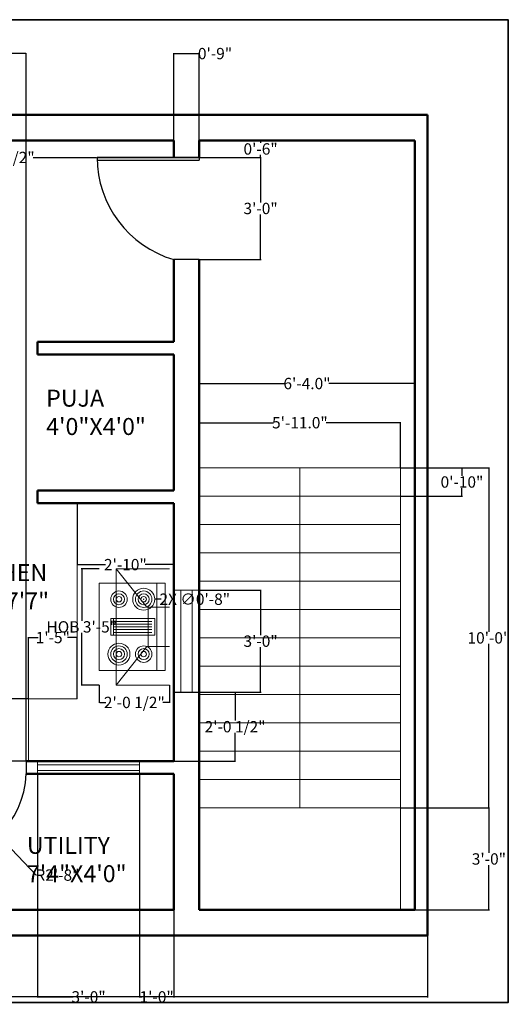
# Model space of a CAD drawing. Units: inches. Extents: x 124 to 591, y 365 to 713.
# Tile 5 of 5: x 418 to 591, y 365 to 713. Entities that reach past the tile are written whole.
import ezdxf

# ---------------------------------------------------------------- set-up
doc = ezdxf.new("R2010")
doc.units = ezdxf.units.IN
doc.header["$MEASUREMENT"] = 0
for name, color, linetype, lineweight in [('A-ANNO-DIMS', 2, 'Continuous', 18), ('A-ANNO-TTLB', 7, 'Continuous', 35), ('A-AREA-IDEN', 7, 'Continuous', 25), ('A-DOOR', 4, 'Continuous', 25), ('A-EQPM', 8, 'Continuous', 18), ('A-FLOR-CASE', 8, 'Continuous', 18), ('A-FLOR-STRS', 7, 'Continuous', 18), ('A-GLAZ', 4, 'Continuous', 18), ('A-WALL', 7, 'Continuous', 50)]:
    doc.layers.add(name, color=color, linetype=linetype, lineweight=lineweight)
doc.styles.get("Standard").update_dxf_attribs({"font": 'arial.ttf'})
doc.dimstyles.get("Standard").update_dxf_attribs({"dimtxt": 4, "dimasz": 0.18, "dimexe": 0.18, "dimexo": 0.0625, "dimgap": 0.09, "dimtad": 0, "dimtih": 1, "dimtoh": 1, "dimdec": 1, "dimzin": 0, "dimdsep": 46, "dimlunit": 3, "dimtxsty": 'Standard', "dimcen": 0.09, "dimclrd": 6, "dimclrt": 3, "dimadec": 0, "dimazin": 0, "dimtfac": 1, "dimtdec": 1, "dimtofl": 0, "dimtmove": 0, "dimatfit": 3, "dimfxl": 1, "dimtfillclr": 6, "dimtolj": 1, "dimtzin": 0, "dimarcsym": 0})

# ---------------------------------------------------------------- blocks, each defined once
blk = doc.blocks.new('chimmne')
for p, q in [((17.89, 6.07), (-18.11, 6.07)), ((-18.11, 6.07), (-18.11, -10.43)), ((-6.16, -3.43), (-18.11, 6.07)), ((5.94, -3.43), (17.89, 6.07)), ((17.89, 6.07), (17.89, -10.43)), ((-6.16, -3.43), (-6.16, -10.43)), ((5.94, -3.82), (-6.16, -3.82)), ((5.94, -3.43), (5.94, -10.43))]:
    blk.add_line(p, q)
for points in [[(-13.61, -9.12), (-13.61, 11.28), (13.39, 11.28), (13.39, -9.12)], [(-2.66, -5.87), (-2.66, 7.73), (2.44, 7.73), (2.44, -5.87)]]:
    blk.add_lwpolyline(points, close=True)
for points in [[(-2.66, 6.88), (2.44, 6.88)], [(-1.81, 6.88), (-1.81, -5.02)], [(-0.96, -5.02), (-0.96, 6.88)], [(-0.11, 6.88), (-0.11, -5.02)], [(0.74, -5.02), (0.74, 6.88)], [(1.59, 6.88), (1.59, -5.02)], [(13.39, -6.57), (-13.61, -6.57)]]:
    blk.add_lwpolyline(points)
for centre, radius in [((-8.55, 5.18), 3.4), ((-8.55, 5.18), 2.55), ((-8.55, 5.18), 1.7), ((8.44, 5.18), 2.55), ((8.44, 5.18), 1.7), ((-8.55, 5.18), 0.85), ((8.44, 5.18), 0.85), ((-8.55, -2.47), 2.55), ((8.44, -2.47), 3.4), ((8.44, -2.47), 2.55), ((-8.55, -2.47), 1.7), ((-8.55, -2.47), 0.85), ((8.44, -2.47), 1.7), ((8.44, -2.47), 0.85)]:
    blk.add_circle(centre, radius)
blk = doc.blocks.new('*D22')
at = {"layer": 'A-ANNO-DIMS', "color": 0, "lineweight": -2, "transparency": 16777216}
for p, q in [((481.64, 554.65), (481.64, 570.69)), ((481.82, 570.51), (507.85, 570.51)), ((552.46, 570.51), (526.43, 570.51)), ((552.64, 554.65), (552.64, 570.69))]:
    blk.add_line(p, q, dxfattribs=at)
at = {"layer": 'A-ANNO-DIMS', "color": 0, "transparency": 16777216}
for points in [[(481.82, 570.54), (481.82, 570.48), (481.64, 570.51)], [(552.46, 570.54), (552.46, 570.48), (552.64, 570.51)]]:
    blk.add_solid(points, dxfattribs=at)
at = {"layer": 'Defpoints', "color": 0, "transparency": 16777216}
for p in [(552.64, 570.51), (481.64, 554.59), (552.64, 554.59)]:
    blk.add_point(p, dxfattribs=at)
at = {"layer": 'A-ANNO-DIMS', "color": 0, "transparency": 16777216, "insert": (517.14, 570.51), "char_height": 4, "attachment_point": 5}
blk.add_mtext('\\A1;5\'-11.0"', dxfattribs=at)
blk = doc.blocks.new('*D23')
at = {"layer": 'A-ANNO-DIMS', "color": 0, "lineweight": -2, "transparency": 16777216}
for p, q in [((481.64, 570.58), (481.64, 584.51)), ((481.82, 584.33), (511.89, 584.33)), ((557.46, 584.33), (527.39, 584.33)), ((557.64, 570.58), (557.64, 584.51))]:
    blk.add_line(p, q, dxfattribs=at)
at = {"layer": 'A-ANNO-DIMS', "color": 0, "transparency": 16777216}
for points in [[(481.82, 584.36), (481.82, 584.3), (481.64, 584.33)], [(557.46, 584.36), (557.46, 584.3), (557.64, 584.33)]]:
    blk.add_solid(points, dxfattribs=at)
at = {"layer": 'Defpoints', "color": 0, "transparency": 16777216}
for p in [(557.64, 584.33), (481.64, 570.51), (557.64, 570.51)]:
    blk.add_point(p, dxfattribs=at)
at = {"layer": 'A-ANNO-DIMS', "color": 0, "transparency": 16777216, "insert": (519.64, 584.33), "char_height": 4, "attachment_point": 5}
blk.add_mtext('\\A1;6\'-4.0"', dxfattribs=at)
blk = doc.blocks.new('*D38')
at = {"layer": 'A-ANNO-DIMS', "color": 0, "lineweight": -2, "transparency": 16777216}
for p, q in [((446.33, 519), (440.06, 519)), ((446.33, 477.96), (440.06, 477.96))]:
    blk.add_line(p, q, dxfattribs=at)
at = {"layer": 'A-ANNO-DIMS', "color": 6, "lineweight": -2, "transparency": 16777216}
for p, q in [((440.24, 518.82), (440.24, 500.64)), ((440.24, 478.14), (440.24, 496.32))]:
    blk.add_line(p, q, dxfattribs=at)
at = {"layer": 'A-ANNO-DIMS', "color": 6, "transparency": 16777216}
for points in [[(440.21, 518.82), (440.27, 518.82), (440.24, 519)], [(440.21, 478.14), (440.27, 478.14), (440.24, 477.96)]]:
    blk.add_solid(points, dxfattribs=at)
at = {"layer": 'Defpoints', "color": 0, "transparency": 16777216}
for p in [(440.24, 519), (446.4, 519), (446.4, 477.96)]:
    blk.add_point(p, dxfattribs=at)
at = {"layer": 'A-ANNO-DIMS', "color": 3, "transparency": 16777216, "insert": (440.24, 498.48), "char_height": 4, "attachment_point": 5}
blk.add_mtext('\\A1;HOB 3\'-5"', dxfattribs=at)
blk = doc.blocks.new('*D39')
at = {"layer": 'A-ANNO-DIMS', "color": 0, "lineweight": -2, "transparency": 16777216}
for p, q in [((446.4, 477.9), (446.4, 471.63)), ((471.14, 477.9), (471.14, 471.63))]:
    blk.add_line(p, q, dxfattribs=at)
at = {"layer": 'A-ANNO-DIMS', "color": 6, "lineweight": -2, "transparency": 16777216}
for p, q in [((446.58, 471.81), (448.67, 471.81)), ((470.96, 471.81), (468.87, 471.81))]:
    blk.add_line(p, q, dxfattribs=at)
at = {"layer": 'A-ANNO-DIMS', "color": 6, "transparency": 16777216}
for points in [[(446.58, 471.84), (446.58, 471.78), (446.4, 471.81)], [(470.96, 471.84), (470.96, 471.78), (471.14, 471.81)]]:
    blk.add_solid(points, dxfattribs=at)
at = {"layer": 'Defpoints', "color": 0, "transparency": 16777216}
for p in [(446.4, 477.96), (471.14, 477.96), (446.4, 471.81)]:
    blk.add_point(p, dxfattribs=at)
at = {"layer": 'A-ANNO-DIMS', "color": 3, "transparency": 16777216, "insert": (458.77, 471.81), "char_height": 4, "attachment_point": 5}
blk.add_mtext('\\A1;2\'-0 1/2"', dxfattribs=at)
blk = doc.blocks.new('*D44')
at = {"layer": 'A-ANNO-DIMS', "color": 0, "lineweight": -2, "transparency": 16777216}
for p, q in [((180.14, 389.53), (180.14, 367.76)), ((562.14, 389.53), (562.14, 367.76))]:
    blk.add_line(p, q, dxfattribs=at)
at = {"layer": 'A-ANNO-DIMS', "color": 6, "lineweight": -2, "transparency": 16777216}
for p, q in [((180.32, 367.94), (362.63, 367.94)), ((561.96, 367.94), (379.65, 367.94))]:
    blk.add_line(p, q, dxfattribs=at)
at = {"layer": 'A-ANNO-DIMS', "color": 6, "transparency": 16777216}
for points in [[(180.32, 367.97), (180.32, 367.91), (180.14, 367.94)], [(561.96, 367.97), (561.96, 367.91), (562.14, 367.94)]]:
    blk.add_solid(points, dxfattribs=at)
at = {"layer": 'Defpoints', "color": 0, "transparency": 16777216}
for p in [(180.14, 389.59), (562.14, 389.59), (562.14, 367.94)]:
    blk.add_point(p, dxfattribs=at)
at = {"layer": 'A-ANNO-DIMS', "color": 3, "transparency": 16777216, "insert": (371.14, 367.94), "char_height": 4, "attachment_point": 5}
blk.add_mtext('\\A1;31\'-10"', dxfattribs=at)
blk = doc.blocks.new('*D45')
at = {"layer": 'A-ANNO-DIMS', "color": 0, "lineweight": -2, "transparency": 16777216}
for p, q in [((552.7, 554.59), (583.97, 554.59)), ((552.7, 434.59), (583.97, 434.59))]:
    blk.add_line(p, q, dxfattribs=at)
at = {"layer": 'A-ANNO-DIMS', "color": 6, "lineweight": -2, "transparency": 16777216}
for p, q in [((583.79, 554.41), (583.79, 496.72)), ((583.79, 434.77), (583.79, 492.46))]:
    blk.add_line(p, q, dxfattribs=at)
at = {"layer": 'A-ANNO-DIMS', "color": 6, "transparency": 16777216}
for points in [[(583.76, 554.41), (583.82, 554.41), (583.79, 554.59)], [(583.76, 434.77), (583.82, 434.77), (583.79, 434.59)]]:
    blk.add_solid(points, dxfattribs=at)
at = {"layer": 'Defpoints', "color": 0, "transparency": 16777216}
for p in [(552.64, 554.59), (583.79, 554.59), (552.64, 434.59)]:
    blk.add_point(p, dxfattribs=at)
at = {"layer": 'A-ANNO-DIMS', "color": 3, "transparency": 16777216, "insert": (583.79, 494.59), "char_height": 4, "attachment_point": 5}
blk.add_mtext('\\A1;10\'-0"', dxfattribs=at)
blk = doc.blocks.new('*D46')
at = {"layer": 'A-ANNO-DIMS', "color": 0, "lineweight": -2, "transparency": 16777216}
for p, q in [((552.7, 554.59), (574.47, 554.59)), ((552.7, 544.59), (574.47, 544.59))]:
    blk.add_line(p, q, dxfattribs=at)
at = {"layer": 'A-ANNO-DIMS', "color": 6, "lineweight": -2, "transparency": 16777216}
for p, q in [((574.29, 554.41), (574.29, 551.72)), ((574.29, 544.77), (574.29, 547.46))]:
    blk.add_line(p, q, dxfattribs=at)
at = {"layer": 'A-ANNO-DIMS', "color": 6, "transparency": 16777216}
for points in [[(574.26, 554.41), (574.32, 554.41), (574.29, 554.59)], [(574.26, 544.77), (574.32, 544.77), (574.29, 544.59)]]:
    blk.add_solid(points, dxfattribs=at)
at = {"layer": 'Defpoints', "color": 0, "transparency": 16777216}
for p in [(552.64, 554.59), (552.64, 544.59), (574.29, 544.59)]:
    blk.add_point(p, dxfattribs=at)
at = {"layer": 'A-ANNO-DIMS', "color": 3, "transparency": 16777216, "insert": (574.29, 549.59), "char_height": 4, "attachment_point": 5}
blk.add_mtext('\\A1;0\'-10"', dxfattribs=at)
blk = doc.blocks.new('*D47')
at = {"layer": 'A-ANNO-DIMS', "color": 0, "lineweight": -2, "transparency": 16777216}
for p, q in [((552.7, 434.59), (583.97, 434.59)), ((552.7, 398.59), (583.97, 398.59))]:
    blk.add_line(p, q, dxfattribs=at)
at = {"layer": 'A-ANNO-DIMS', "color": 6, "lineweight": -2, "transparency": 16777216}
for p, q in [((583.79, 434.41), (583.79, 418.73)), ((583.79, 398.77), (583.79, 414.46))]:
    blk.add_line(p, q, dxfattribs=at)
at = {"layer": 'A-ANNO-DIMS', "color": 6, "transparency": 16777216}
for points in [[(583.76, 434.41), (583.82, 434.41), (583.79, 434.59)], [(583.76, 398.77), (583.82, 398.77), (583.79, 398.59)]]:
    blk.add_solid(points, dxfattribs=at)
at = {"layer": 'Defpoints', "color": 0, "transparency": 16777216}
for p in [(552.64, 434.59), (583.79, 434.59), (552.64, 398.59)]:
    blk.add_point(p, dxfattribs=at)
at = {"layer": 'A-ANNO-DIMS', "color": 3, "transparency": 16777216, "insert": (583.79, 416.59), "char_height": 4, "attachment_point": 5}
blk.add_mtext('\\A1;3\'-0"', dxfattribs=at)
blk = doc.blocks.new('*D49')
at = {"layer": 'A-ANNO-DIMS', "color": 0, "lineweight": -2, "transparency": 16777216}
for p, q in [((481.7, 664.09), (503.47, 664.09)), ((481.7, 628.09), (503.47, 628.09))]:
    blk.add_line(p, q, dxfattribs=at)
at = {"layer": 'A-ANNO-DIMS', "color": 6, "lineweight": -2, "transparency": 16777216}
for p, q in [((503.29, 663.91), (503.29, 648.23)), ((503.29, 628.27), (503.29, 643.96))]:
    blk.add_line(p, q, dxfattribs=at)
at = {"layer": 'A-ANNO-DIMS', "color": 6, "transparency": 16777216}
for points in [[(503.26, 663.91), (503.32, 663.91), (503.29, 664.09)], [(503.26, 628.27), (503.32, 628.27), (503.29, 628.09)]]:
    blk.add_solid(points, dxfattribs=at)
at = {"layer": 'Defpoints', "color": 0, "transparency": 16777216}
for p in [(481.64, 664.09), (481.64, 628.09), (503.29, 628.09)]:
    blk.add_point(p, dxfattribs=at)
at = {"layer": 'A-ANNO-DIMS', "color": 3, "transparency": 16777216, "insert": (503.29, 646.09), "char_height": 4, "attachment_point": 5}
blk.add_mtext('\\A1;3\'-0"', dxfattribs=at)
blk = doc.blocks.new('*D50')
at = {"layer": 'A-ANNO-DIMS', "color": 0, "lineweight": -2, "transparency": 16777216}
for p, q in [((481.7, 670.09), (503.47, 670.09)), ((481.7, 664.09), (503.47, 664.09))]:
    blk.add_line(p, q, dxfattribs=at)
at = {"layer": 'A-ANNO-DIMS', "color": 6, "lineweight": -2, "transparency": 16777216}
for p, q in [((503.29, 669.91), (503.29, 669.22)), ((503.29, 664.27), (503.29, 664.96))]:
    blk.add_line(p, q, dxfattribs=at)
at = {"layer": 'A-ANNO-DIMS', "color": 6, "transparency": 16777216}
for points in [[(503.26, 669.91), (503.32, 669.91), (503.29, 670.09)], [(503.26, 664.27), (503.32, 664.27), (503.29, 664.09)]]:
    blk.add_solid(points, dxfattribs=at)
at = {"layer": 'Defpoints', "color": 0, "transparency": 16777216}
for p in [(481.64, 670.09), (481.64, 664.09), (503.29, 664.09)]:
    blk.add_point(p, dxfattribs=at)
at = {"layer": 'A-ANNO-DIMS', "color": 3, "transparency": 16777216, "insert": (503.29, 667.09), "char_height": 4, "attachment_point": 5}
blk.add_mtext('\\A1;0\'-6"', dxfattribs=at)
blk = doc.blocks.new('*D51')
at = {"layer": 'A-ANNO-DIMS', "color": 0, "lineweight": -2, "transparency": 16777216}
for p, q in [((424.64, 446.53), (424.64, 367.76)), ((460.64, 446.53), (460.64, 367.76))]:
    blk.add_line(p, q, dxfattribs=at)
at = {"layer": 'A-ANNO-DIMS', "color": 6, "lineweight": -2, "transparency": 16777216}
for p, q in [((424.82, 367.94), (437.23, 367.94)), ((460.46, 367.94), (448.04, 367.94))]:
    blk.add_line(p, q, dxfattribs=at)
at = {"layer": 'A-ANNO-DIMS', "color": 6, "transparency": 16777216}
for points in [[(424.82, 367.97), (424.82, 367.91), (424.64, 367.94)], [(460.46, 367.97), (460.46, 367.91), (460.64, 367.94)]]:
    blk.add_solid(points, dxfattribs=at)
at = {"layer": 'Defpoints', "color": 0, "transparency": 16777216}
for p in [(424.64, 446.59), (460.64, 446.59), (460.64, 367.94)]:
    blk.add_point(p, dxfattribs=at)
at = {"layer": 'A-ANNO-DIMS', "color": 3, "transparency": 16777216, "insert": (442.64, 367.94), "char_height": 4, "attachment_point": 5}
blk.add_mtext('\\A1;3\'-0"', dxfattribs=at)
blk = doc.blocks.new('*D52')
at = {"layer": 'A-ANNO-DIMS', "color": 0, "lineweight": -2, "transparency": 16777216}
for p, q in [((460.64, 446.53), (460.64, 367.76)), ((472.64, 446.53), (472.64, 367.76))]:
    blk.add_line(p, q, dxfattribs=at)
at = {"layer": 'A-ANNO-DIMS', "color": 6, "lineweight": -2, "transparency": 16777216}
for p, q in [((460.82, 367.94), (461.42, 367.94)), ((472.46, 367.94), (471.86, 367.94))]:
    blk.add_line(p, q, dxfattribs=at)
at = {"layer": 'A-ANNO-DIMS', "color": 6, "transparency": 16777216}
for points in [[(460.82, 367.97), (460.82, 367.91), (460.64, 367.94)], [(472.46, 367.97), (472.46, 367.91), (472.64, 367.94)]]:
    blk.add_solid(points, dxfattribs=at)
at = {"layer": 'Defpoints', "color": 0, "transparency": 16777216}
for p in [(460.64, 446.59), (472.64, 446.59), (472.64, 367.94)]:
    blk.add_point(p, dxfattribs=at)
at = {"layer": 'A-ANNO-DIMS', "color": 3, "transparency": 16777216, "insert": (466.64, 367.94), "char_height": 4, "attachment_point": 5}
blk.add_mtext('\\A1;1\'-0"', dxfattribs=at)
blk = doc.blocks.new('*D53')
at = {"layer": 'A-ANNO-DIMS', "color": 0, "lineweight": -2, "transparency": 16777216}
for p, q in [((481.7, 511.43), (503.47, 511.43)), ((481.7, 475.43), (503.47, 475.43))]:
    blk.add_line(p, q, dxfattribs=at)
at = {"layer": 'A-ANNO-DIMS', "color": 6, "lineweight": -2, "transparency": 16777216}
for p, q in [((503.29, 511.25), (503.29, 495.57)), ((503.29, 475.61), (503.29, 491.3))]:
    blk.add_line(p, q, dxfattribs=at)
at = {"layer": 'A-ANNO-DIMS', "color": 6, "transparency": 16777216}
for points in [[(503.26, 511.25), (503.32, 511.25), (503.29, 511.43)], [(503.26, 475.61), (503.32, 475.61), (503.29, 475.43)]]:
    blk.add_solid(points, dxfattribs=at)
at = {"layer": 'Defpoints', "color": 0, "transparency": 16777216}
for p in [(481.64, 511.43), (481.64, 475.43), (503.29, 475.43)]:
    blk.add_point(p, dxfattribs=at)
at = {"layer": 'A-ANNO-DIMS', "color": 3, "transparency": 16777216, "insert": (503.29, 493.43), "char_height": 4, "attachment_point": 5}
blk.add_mtext('\\A1;3\'-0"', dxfattribs=at)
blk = doc.blocks.new('*D54')
at = {"layer": 'A-ANNO-DIMS', "color": 0, "lineweight": -2, "transparency": 16777216}
for p, q in [((472.7, 475.43), (494.47, 475.43)), ((472.7, 451.09), (494.47, 451.09))]:
    blk.add_line(p, q, dxfattribs=at)
at = {"layer": 'A-ANNO-DIMS', "color": 6, "lineweight": -2, "transparency": 16777216}
for p, q in [((494.29, 475.25), (494.29, 465.42)), ((494.29, 451.27), (494.29, 461.1))]:
    blk.add_line(p, q, dxfattribs=at)
at = {"layer": 'A-ANNO-DIMS', "color": 6, "transparency": 16777216}
for points in [[(494.26, 475.25), (494.32, 475.25), (494.29, 475.43)], [(494.26, 451.27), (494.32, 451.27), (494.29, 451.09)]]:
    blk.add_solid(points, dxfattribs=at)
at = {"layer": 'Defpoints', "color": 0, "transparency": 16777216}
for p in [(472.64, 475.43), (472.64, 451.09), (494.29, 451.09)]:
    blk.add_point(p, dxfattribs=at)
at = {"layer": 'A-ANNO-DIMS', "color": 3, "transparency": 16777216, "insert": (494.29, 463.26), "char_height": 4, "attachment_point": 5}
blk.add_mtext('\\A1;2\'-0 1/2"', dxfattribs=at)
blk = doc.blocks.new('*D57')
at = {"layer": 'A-ANNO-DIMS', "color": 0, "lineweight": -2, "transparency": 16777216}
for p, q in [((388.64, 451.15), (388.64, 700.92)), ((420.64, 451.15), (420.64, 700.92))]:
    blk.add_line(p, q, dxfattribs=at)
at = {"layer": 'A-ANNO-DIMS', "color": 6, "lineweight": -2, "transparency": 16777216}
for p, q in [((388.82, 700.74), (399.2, 700.74)), ((420.46, 700.74), (410.08, 700.74))]:
    blk.add_line(p, q, dxfattribs=at)
at = {"layer": 'A-ANNO-DIMS', "color": 6, "transparency": 16777216}
for points in [[(388.82, 700.77), (388.82, 700.71), (388.64, 700.74)], [(420.46, 700.77), (420.46, 700.71), (420.64, 700.74)]]:
    blk.add_solid(points, dxfattribs=at)
at = {"layer": 'Defpoints', "color": 0, "transparency": 16777216}
for p in [(420.64, 700.74), (388.64, 451.09), (420.64, 451.09)]:
    blk.add_point(p, dxfattribs=at)
at = {"layer": 'A-ANNO-DIMS', "color": 3, "transparency": 16777216, "insert": (404.64, 700.74), "char_height": 4, "attachment_point": 5}
blk.add_mtext('\\A1;2\'-8"', dxfattribs=at)
blk = doc.blocks.new('*D58')
at = {"layer": 'A-ANNO-DIMS', "color": 0, "lineweight": -2, "transparency": 16777216}
for p, q in [((472.64, 670.15), (472.64, 700.92)), ((481.64, 670.15), (481.64, 700.92))]:
    blk.add_line(p, q, dxfattribs=at)
at = {"layer": 'A-ANNO-DIMS', "color": 6, "lineweight": -2, "transparency": 16777216}
for p, q in [((472.82, 700.74), (481.46, 700.74)), ((481.64, 700.74), (481.82, 700.74))]:
    blk.add_line(p, q, dxfattribs=at)
at = {"layer": 'A-ANNO-DIMS', "color": 6, "transparency": 16777216}
for points in [[(472.82, 700.77), (472.82, 700.71), (472.64, 700.74)], [(481.46, 700.77), (481.46, 700.71), (481.64, 700.74)]]:
    blk.add_solid(points, dxfattribs=at)
at = {"layer": 'Defpoints', "color": 0, "transparency": 16777216}
for p in [(481.64, 700.74), (472.64, 670.09), (481.64, 670.09)]:
    blk.add_point(p, dxfattribs=at)
at = {"layer": 'A-ANNO-DIMS', "color": 3, "transparency": 16777216, "insert": (487.22, 700.74), "char_height": 4, "attachment_point": 5}
blk.add_mtext('\\A1;0\'-9"', dxfattribs=at)
blk = doc.blocks.new('*D62')
at = {"layer": 'A-ANNO-DIMS', "color": 0, "lineweight": -2, "transparency": 16777216}
for p, q in [((438.57, 542.03), (438.57, 520.26)), ((472.64, 542.03), (472.64, 520.26))]:
    blk.add_line(p, q, dxfattribs=at)
at = {"layer": 'A-ANNO-DIMS', "color": 6, "lineweight": -2, "transparency": 16777216}
for p, q in [((438.75, 520.44), (448.61, 520.44)), ((472.46, 520.44), (462.6, 520.44))]:
    blk.add_line(p, q, dxfattribs=at)
at = {"layer": 'A-ANNO-DIMS', "color": 6, "transparency": 16777216}
for points in [[(438.75, 520.47), (438.75, 520.41), (438.57, 520.44)], [(472.46, 520.47), (472.46, 520.41), (472.64, 520.44)]]:
    blk.add_solid(points, dxfattribs=at)
at = {"layer": 'Defpoints', "color": 0, "transparency": 16777216}
for p in [(438.57, 542.09), (472.64, 542.09), (438.57, 520.44)]:
    blk.add_point(p, dxfattribs=at)
at = {"layer": 'A-ANNO-DIMS', "color": 3, "transparency": 16777216, "insert": (455.61, 520.44), "char_height": 4, "attachment_point": 5}
blk.add_mtext('\\A1;2\'-10"', dxfattribs=at)
blk = doc.blocks.new('*D63')
at = {"layer": 'A-ANNO-DIMS', "color": 0, "lineweight": -2, "transparency": 16777216}
for p, q in [((421.5, 473.13), (421.5, 494.9)), ((438.57, 473.13), (438.57, 494.9))]:
    blk.add_line(p, q, dxfattribs=at)
at = {"layer": 'A-ANNO-DIMS', "color": 6, "lineweight": -2, "transparency": 16777216}
for p, q in [((421.68, 494.72), (424.82, 494.72)), ((438.39, 494.72), (435.25, 494.72))]:
    blk.add_line(p, q, dxfattribs=at)
at = {"layer": 'A-ANNO-DIMS', "color": 6, "transparency": 16777216}
for points in [[(421.68, 494.75), (421.68, 494.69), (421.5, 494.72)], [(438.39, 494.75), (438.39, 494.69), (438.57, 494.72)]]:
    blk.add_solid(points, dxfattribs=at)
at = {"layer": 'Defpoints', "color": 0, "transparency": 16777216}
for p in [(438.57, 494.72), (421.5, 473.07), (438.57, 473.07)]:
    blk.add_point(p, dxfattribs=at)
at = {"layer": 'A-ANNO-DIMS', "color": 3, "transparency": 16777216, "insert": (430.03, 494.72), "char_height": 4, "attachment_point": 5}
blk.add_mtext('\\A1;1\'-5"', dxfattribs=at)
blk = doc.blocks.new('*D64')
at = {"layer": 'A-ANNO-DIMS', "color": 0, "lineweight": -2, "transparency": 16777216}
for p, q in [((421.43, 473.07), (399.67, 473.07)), ((421.43, 451.09), (399.67, 451.09))]:
    blk.add_line(p, q, dxfattribs=at)
at = {"layer": 'A-ANNO-DIMS', "color": 6, "lineweight": -2, "transparency": 16777216}
for p, q in [((399.85, 472.89), (399.85, 464.21)), ((399.85, 451.27), (399.85, 459.95))]:
    blk.add_line(p, q, dxfattribs=at)
at = {"layer": 'A-ANNO-DIMS', "color": 6, "transparency": 16777216}
for points in [[(399.82, 472.89), (399.88, 472.89), (399.85, 473.07)], [(399.82, 451.27), (399.88, 451.27), (399.85, 451.09)]]:
    blk.add_solid(points, dxfattribs=at)
at = {"layer": 'Defpoints', "color": 0, "transparency": 16777216}
for p in [(399.85, 473.07), (421.5, 473.07), (421.5, 451.09)]:
    blk.add_point(p, dxfattribs=at)
at = {"layer": 'A-ANNO-DIMS', "color": 3, "transparency": 16777216, "insert": (399.85, 462.08), "char_height": 4, "attachment_point": 5}
blk.add_mtext('\\A1;1\'-10"', dxfattribs=at)
blk = doc.blocks.new('*D69')
at = {"layer": 'A-ANNO-DIMS', "color": 0, "lineweight": -2, "transparency": 16777216}
for p, q in [((388.55, 447.85), (388.73, 447.85)), ((388.64, 447.76), (388.64, 447.94))]:
    blk.add_line(p, q, dxfattribs=at)
at = {"layer": 'A-ANNO-DIMS', "color": 6, "lineweight": -2, "transparency": 16777216}
for p, q in [((424.15, 410.91), (410.96, 424.64)), ((424.33, 410.91), (424.15, 410.91))]:
    blk.add_line(p, q, dxfattribs=at)
at = {"layer": 'A-ANNO-DIMS', "color": 6, "transparency": 16777216}
blk.add_solid([(410.98, 424.66), (410.94, 424.62), (410.83, 424.77)], dxfattribs=at)
at = {"layer": 'Defpoints', "color": 0, "transparency": 16777216}
for p in [(388.64, 447.85), (410.83, 424.77)]:
    blk.add_point(p, dxfattribs=at)
at = {"layer": 'A-ANNO-DIMS', "color": 3, "transparency": 16777216, "insert": (431.65, 410.91), "char_height": 4, "attachment_point": 5}
blk.add_mtext('\\A1;R2\'-8"', dxfattribs=at)
blk = doc.blocks.new('*D71')
at = {"layer": 'A-ANNO-DIMS', "color": 6, "lineweight": -2, "transparency": 16777216}
blk.add_line((423.14, 664.09), (445.46, 664.09), dxfattribs=at)
at = {"layer": 'A-ANNO-DIMS', "color": 0, "lineweight": -2, "transparency": 16777216}
for p, q in [((483.05, 664.09), (483.23, 664.09)), ((483.14, 664), (483.14, 664.18))]:
    blk.add_line(p, q, dxfattribs=at)
at = {"layer": 'A-ANNO-DIMS', "color": 6, "transparency": 16777216}
blk.add_solid([(445.46, 664.12), (445.46, 664.06), (445.64, 664.09)], dxfattribs=at)
at = {"layer": 'Defpoints', "color": 0, "transparency": 16777216}
for p in [(445.64, 664.09), (483.14, 664.09)]:
    blk.add_point(p, dxfattribs=at)
at = {"layer": 'A-ANNO-DIMS', "color": 3, "transparency": 16777216, "insert": (411.16, 664.09), "char_height": 4, "attachment_point": 5}
blk.add_mtext('\\A1;R3\'-1 1/2"', dxfattribs=at)
blk = doc.blocks.new('*D73')
at = {"layer": 'A-ANNO-DIMS', "color": 0, "lineweight": -2, "transparency": 16777216}
for p, q in [((461.98, 508.24), (462.16, 508.24)), ((462.07, 508.15), (462.07, 508.33))]:
    blk.add_line(p, q, dxfattribs=at)
at = {"layer": 'A-ANNO-DIMS', "color": 6, "lineweight": -2, "transparency": 16777216}
blk.add_line((468.27, 508.24), (466.13, 508.24), dxfattribs=at)
at = {"layer": 'A-ANNO-DIMS', "color": 6, "transparency": 16777216}
blk.add_solid([(466.13, 508.27), (466.13, 508.21), (465.95, 508.24)], dxfattribs=at)
at = {"layer": 'Defpoints', "color": 0, "transparency": 16777216}
for p in [(458.2, 508.24), (465.95, 508.24)]:
    blk.add_point(p, dxfattribs=at)
at = {"layer": 'A-ANNO-DIMS', "color": 3, "transparency": 16777216, "insert": (480.08, 508.24), "char_height": 4, "attachment_point": 5}
blk.add_mtext('\\A1;2X ∅0\'-8"', dxfattribs=at)

msp = doc.modelspace()

# ---------------------------------------------------------------- linework, layer by layer
at = {"layer": 'A-ANNO-TTLB'}
msp.add_lwpolyline([(124.09, 712.7), (590.57, 712.7), (590.57, 365.95), (124.09, 365.95)], close=True, dxfattribs=at)
msp.add_lwpolyline([(124.09, 712.7), (590.57, 712.7), (590.57, 365.95), (124.09, 365.95)], close=True, dxfattribs=at)
at = {"layer": 'A-DOOR'}
for p, q in [((481.64, 664.09), (445.64, 664.09)), ((445.64, 664.09), (481.64, 664.09)), ((481.64, 664.09), (481.64, 663.09)), ((445.64, 663.09), (481.64, 663.09)), ((481.64, 628.09), (472.64, 628.09)), ((420.64, 451.09), (420.64, 446.59))]:
    msp.add_line(p, q, dxfattribs=at)
for centre, radius, start, end in [((483.14, 664.09), 37.5, 180, 253.7398), ((388.64, 447.85), 32.02, 270, 357.7413)]:
    msp.add_arc(centre, radius, start, end, dxfattribs=at)
at = {"layer": 'A-FLOR-CASE'}
for p, q in [((438.57, 542.09), (438.57, 473.07)), ((438.57, 473.07), (421.5, 473.07)), ((421.5, 473.07), (421.5, 451.09))]:
    msp.add_line(p, q, dxfattribs=at)
at = {"layer": 'A-FLOR-STRS'}
for p, q in [((481.64, 554.59), (552.64, 554.59)), ((517.14, 554.59), (517.14, 434.59)), ((552.64, 434.59), (552.64, 554.59)), ((481.64, 544.59), (552.64, 544.59)), ((481.64, 534.59), (552.64, 534.59)), ((481.64, 524.59), (552.64, 524.59)), ((481.64, 514.59), (552.64, 514.59)), ((481.64, 504.59), (552.64, 504.59)), ((481.64, 494.59), (552.64, 494.59)), ((481.64, 484.59), (552.64, 484.59)), ((481.64, 474.59), (552.64, 474.59)), ((481.64, 464.59), (552.64, 464.59)), ((481.64, 454.59), (552.64, 454.59)), ((481.64, 444.59), (552.64, 444.59)), ((481.64, 398.59), (481.64, 434.59)), ((481.64, 434.59), (481.64, 434.59)), ((481.64, 434.59), (552.64, 434.59)), ((552.64, 434.59), (552.64, 398.59))]:
    msp.add_line(p, q, dxfattribs=at)
at = {"layer": 'A-GLAZ'}
for p, q in [((472.64, 511.43), (481.64, 511.43)), ((475.14, 511.43), (475.14, 475.43)), ((481.64, 511.43), (477.14, 511.43)), ((479.14, 511.43), (479.14, 475.43)), ((477.14, 475.43), (472.64, 475.43)), ((472.64, 475.43), (481.64, 475.43)), ((424.64, 448.84), (424.64, 451.09)), ((424.64, 451.09), (424.64, 446.59)), ((460.64, 449.84), (424.64, 449.84)), ((460.64, 446.59), (460.64, 451.09)), ((460.64, 451.09), (460.64, 448.84)), ((460.64, 447.84), (424.64, 447.84))]:
    msp.add_line(p, q, dxfattribs=at)
at = {"layer": 'A-WALL'}
for p, q in [((180.14, 679.09), (562.14, 679.09)), ((562.14, 679.09), (562.14, 389.59)), ((301.64, 670.09), (472.64, 670.09)), ((472.64, 670.09), (472.64, 664.09)), ((481.64, 670.09), (481.64, 664.09)), ((481.64, 670.09), (481.64, 664.09)), ((481.64, 670.09), (557.64, 670.09)), ((557.64, 670.09), (557.64, 398.59)), ((472.64, 628.09), (472.64, 599.09)), ((481.64, 628.09), (481.64, 398.59)), ((424.64, 599.09), (472.64, 599.09)), ((424.64, 599.09), (424.64, 594.59)), ((424.64, 594.59), (472.64, 594.59)), ((472.64, 594.59), (472.64, 546.59)), ((424.64, 546.59), (424.64, 542.09)), ((424.64, 546.59), (472.64, 546.59)), ((424.64, 542.09), (472.64, 542.09)), ((472.64, 542.09), (472.64, 451.09)), ((420.64, 451.09), (472.64, 451.09)), ((420.64, 446.59), (472.64, 446.59)), ((472.64, 446.59), (460.64, 446.59)), ((472.64, 446.59), (472.64, 398.59)), ((385.64, 398.59), (472.64, 398.59)), ((481.64, 398.59), (557.64, 398.59)), ((180.14, 389.59), (562.14, 389.59))]:
    msp.add_line(p, q, dxfattribs=at)

# ---------------------------------------------------------------- block references
at = {"layer": 'A-EQPM', "xscale": 1.14, "yscale": 1.14, "zscale": 1.14, "rotation": 89.99999999997907}
msp.add_blockref('chimmne', (459.25, 498.61), dxfattribs=at)

# ---------------------------------------------------------------- texts
at = {"layer": 'A-AREA-IDEN', "char_height": 6, "attachment_point": 1}
for s, width, insert in [('PUJA\\P4\'0"X4\'0"', 40.34, (427.68, 582.17)), ('KITCHEN\\P7\'4"X7\'7"', 40.647, (393.54, 520.61)), ('UTILITY\\P7\'4"X4\'0"', 40.5799, (420.88, 424.4))]:
    msp.add_mtext_dynamic_manual_height_columns(s, width=width, gutter_width=1, heights=[0], dxfattribs=dict(at, insert=insert))

# ---------------------------------------------------------------- dimensions: what is measured, and where the dimension line sits
at = {"layer": 'A-ANNO-DIMS'}
for base, p1, p2, override, picture, middle in [((420.64, 700.74), (388.64, 451.09), (420.64, 451.09), {"dimdec": 1, "dimlfac": 1, "dimrnd": 0, "dimzin": 1, "dimdsep": 46, "dimlunit": 4, "dimfrac": 2}, '*D57', (404.64, 700.74)), ((481.64, 700.74), (472.64, 670.09), (481.64, 670.09), {"dimdec": 1, "dimlfac": 1, "dimrnd": 0, "dimzin": 1, "dimdsep": 46, "dimlunit": 4, "dimfrac": 2}, '*D58', (487.22, 700.74)), ((557.64, 584.33), (481.64, 570.51), (557.64, 570.51), {"dimclrd": 0, "dimclre": 0, "dimclrt": 0}, '*D23', (519.64, 584.33)), ((552.64, 570.51), (481.64, 554.59), (552.64, 554.59), {"dimclrd": 0, "dimclre": 0, "dimclrt": 0}, '*D22', (517.14, 570.51)), ((438.57, 494.72), (421.5, 473.07), (438.57, 473.07), {"dimdec": 1, "dimlfac": 1, "dimrnd": 0, "dimzin": 1, "dimdsep": 46, "dimlunit": 4, "dimfrac": 2}, '*D63', (430.03, 494.72)), ((460.64, 367.94), (424.64, 446.59), (460.64, 446.59), {"dimdec": 1, "dimlfac": 1, "dimrnd": 0, "dimzin": 1, "dimdsep": 46, "dimlunit": 4, "dimfrac": 2}, '*D51', (442.64, 367.94)), ((472.64, 367.94), (460.64, 446.59), (472.64, 446.59), {"dimdec": 1, "dimlfac": 1, "dimrnd": 0, "dimzin": 1, "dimdsep": 46, "dimlunit": 4, "dimfrac": 2}, '*D52', (466.64, 367.94)), ((562.14, 367.94), (180.14, 389.59), (562.14, 389.59), {"dimdec": 1, "dimlfac": 1, "dimrnd": 0, "dimzin": 1, "dimdsep": 46, "dimlunit": 4, "dimfrac": 2}, '*D44', (371.14, 367.94))]:
    dim = msp.add_linear_dim(base=base, p1=p1, p2=p2, dimstyle='Standard', override=override, dxfattribs=at)
    dim.commit()
    dim.dimension.update_dxf_attribs({"geometry": picture, "text_midpoint": middle})
for center, mpoint, picture, middle in [((483.14, 664.09), (445.64, 664.09), '*D71', (423.14, 664.09)), ((388.64, 447.85), (410.83, 424.77), '*D69', (431.65, 410.91))]:
    dim = msp.add_radius_dim(center=center, mpoint=mpoint, dimstyle='Standard', override={"dimdec": 1, "dimlfac": 1, "dimrnd": 0, "dimzin": 1, "dimdsep": 46, "dimlunit": 4, "dimfrac": 2}, dxfattribs=at)
    dim.commit()
    dim.dimension.update_dxf_attribs({"geometry": picture, "text_midpoint": middle, "dimtype": 164})
for base, p1, p2, angle, picture, middle in [((503.29, 664.09), (481.64, 670.09), (481.64, 664.09), 270, '*D50', (503.29, 667.09)), ((503.29, 628.09), (481.64, 664.09), (481.64, 628.09), 270, '*D49', (503.29, 646.09)), ((583.79, 554.59), (552.64, 434.59), (552.64, 554.59), 90, '*D45', (583.79, 494.59)), ((574.29, 544.59), (552.64, 554.59), (552.64, 544.59), 270, '*D46', (574.29, 549.59)), ((438.57, 520.44), (472.64, 542.09), (438.57, 542.09), 180, '*D62', (455.61, 520.44)), ((503.29, 475.43), (481.64, 511.43), (481.64, 475.43), 270, '*D53', (503.29, 493.43)), ((446.4, 471.81), (471.14, 477.96), (446.4, 477.96), 180, '*D39', (458.77, 471.81)), ((399.85, 473.07), (421.5, 451.09), (421.5, 473.07), 90, '*D64', (399.85, 462.08)), ((494.29, 451.09), (472.64, 475.43), (472.64, 451.09), 270, '*D54', (494.29, 463.26)), ((583.79, 434.59), (552.64, 398.59), (552.64, 434.59), 90, '*D47', (583.79, 416.59))]:
    dim = msp.add_linear_dim(base=base, p1=p1, p2=p2, angle=angle, dimstyle='Standard', override={"dimdec": 1, "dimlfac": 1, "dimrnd": 0, "dimzin": 1, "dimdsep": 46, "dimlunit": 4, "dimfrac": 2}, dxfattribs=at)
    dim.commit()
    dim.dimension.update_dxf_attribs({"geometry": picture, "text_midpoint": middle})
dim = msp.add_linear_dim(base=(440.24, 519), p1=(446.4, 477.96), p2=(446.4, 519), angle=90, text='HOB <>', dimstyle='Standard', override={"dimdec": 1, "dimlfac": 1, "dimrnd": 0, "dimzin": 1, "dimdsep": 46, "dimlunit": 4, "dimfrac": 2}, dxfattribs=at)
dim.commit()
dim.dimension.update_dxf_attribs({"geometry": '*D38', "text_midpoint": (440.24, 498.48)})
dim = msp.add_diameter_dim_2p(p1=(458.1959, 508.2379), p2=(465.9479, 508.237), text='2X <>', dimstyle='Standard', override={"dimdec": 1, "dimlfac": 1, "dimrnd": 0, "dimzin": 1, "dimdsep": 46, "dimlunit": 4, "dimfrac": 2}, dxfattribs=at)
dim.commit()
dim.dimension.update_dxf_attribs({"geometry": '*D73', "text_midpoint": (468.2735, 508.2367), "dimtype": 163})

doc.saveas('drawing.dxf')
